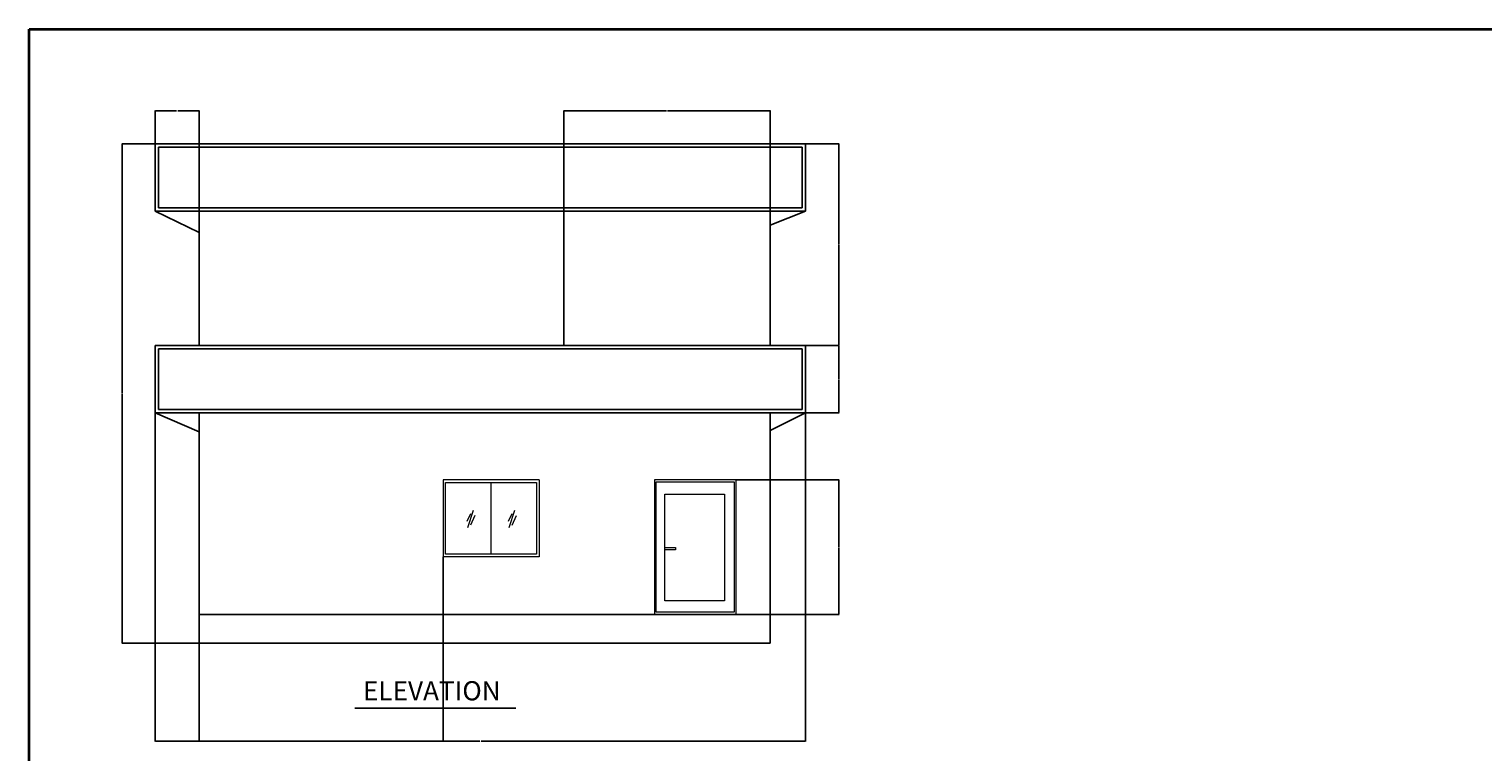
# Model space of a CAD drawing. Units: inches. Extents: x 1912 to 3731, y 1384 to 2459.
# Tile 5 of 8: x 1912 to 2821, y 2007 to 2459. Entities that reach past the tile are written whole.
import ezdxf

# ---------------------------------------------------------------- set-up
doc = ezdxf.new("R2010")
doc.units = ezdxf.units.IN
for name, color, linetype, lineweight in [('A-ANNO-DIMS', 2, 'Continuous', 18), ('A-ANNO-TITL', 7, 'Continuous', 25), ('A-ANNO-TTLB', 7, 'Continuous', 35), ('A-DOOR', 3, 'Continuous', 20), ('A-ELEV', 7, 'Continuous', 25), ('A-GLAZ', 4, 'Continuous', 18)]:
    doc.layers.add(name, color=color, linetype=linetype, lineweight=lineweight)
doc.styles.get("Standard").update_dxf_attribs({"font": 'arial.ttf'})
doc.dimstyles.get("Standard").update_dxf_attribs({"dimtxt": 0.18, "dimasz": 0.18, "dimexe": 0.18, "dimexo": 0.0625, "dimgap": 0.09, "dimtad": 0, "dimtih": 1, "dimtoh": 1, "dimdec": 4, "dimzin": 0, "dimdsep": 46, "dimtxsty": 'Standard', "dimcen": 0.09, "dimadec": 0, "dimazin": 0, "dimtfac": 1, "dimtdec": 4, "dimtofl": 0, "dimtmove": 0, "dimatfit": 3, "dimfxl": 1, "dimtolj": 1, "dimtzin": 0, "dimarcsym": 0})

# ---------------------------------------------------------------- blocks, each defined once
blk = doc.blocks.new('*D115')
at = {"layer": 'A-ANNO-DIMS', "color": 0, "lineweight": -2, "transparency": 16777216}
for p, q in [((1991.12, 2218.67), (1991.12, 2013.22)), ((2397.55, 2218.67), (2397.55, 2013.22)), ((1991.3, 2013.4), (2193.94, 2013.4)), ((2397.37, 2013.4), (2194.73, 2013.4))]:
    blk.add_line(p, q, dxfattribs=at)
at = {"layer": 'A-ANNO-DIMS', "color": 0, "transparency": 16777216}
for points in [[(1991.3, 2013.43), (1991.3, 2013.37), (1991.12, 2013.4)], [(2397.37, 2013.43), (2397.37, 2013.37), (2397.55, 2013.4)]]:
    blk.add_solid(points, dxfattribs=at)
at = {"layer": 'Defpoints', "color": 0, "transparency": 16777216}
for p in [(1991.12, 2218.73), (2397.55, 2218.73), (2397.55, 2013.4)]:
    blk.add_point(p, dxfattribs=at)
at = {"layer": 'A-ANNO-DIMS', "color": 0, "transparency": 16777216, "insert": (2194.33, 2013.4), "char_height": 0.18, "attachment_point": 5}
blk.add_mtext('\\A1;406.4', dxfattribs=at)
blk = doc.blocks.new('*D116')
at = {"layer": 'A-ANNO-DIMS', "color": 0, "lineweight": -2, "transparency": 16777216}
for p, q in [((1991.05, 2386.73), (1970.19, 2386.73)), ((1970.37, 2386.55), (1970.37, 2230.92)), ((1970.37, 2074.91), (1970.37, 2230.55)), ((2018.47, 2074.73), (1970.19, 2074.73))]:
    blk.add_line(p, q, dxfattribs=at)
at = {"layer": 'A-ANNO-DIMS', "color": 0, "transparency": 16777216}
for points in [[(1970.34, 2386.55), (1970.4, 2386.55), (1970.37, 2386.73)], [(1970.34, 2074.91), (1970.4, 2074.91), (1970.37, 2074.73)]]:
    blk.add_solid(points, dxfattribs=at)
at = {"layer": 'Defpoints', "color": 0, "transparency": 16777216}
for p in [(1970.37, 2386.73), (1991.12, 2386.73), (2018.53, 2074.73)]:
    blk.add_point(p, dxfattribs=at)
at = {"layer": 'A-ANNO-DIMS', "color": 0, "transparency": 16777216, "insert": (1970.37, 2230.73), "char_height": 0.18, "attachment_point": 5}
blk.add_mtext('\\A1;312', dxfattribs=at)
blk = doc.blocks.new('*D117')
at = {"layer": 'A-ANNO-DIMS', "color": 0, "lineweight": -2, "transparency": 16777216}
for p, q in [((2171, 2128.67), (2171, 2013.22)), ((2018.53, 2092.67), (2018.53, 2013.22)), ((2018.71, 2013.4), (2094.31, 2013.4)), ((2170.82, 2013.4), (2095.22, 2013.4))]:
    blk.add_line(p, q, dxfattribs=at)
at = {"layer": 'A-ANNO-DIMS', "color": 0, "transparency": 16777216}
for points in [[(2018.71, 2013.43), (2018.71, 2013.37), (2018.53, 2013.4)], [(2170.82, 2013.43), (2170.82, 2013.37), (2171, 2013.4)]]:
    blk.add_solid(points, dxfattribs=at)
at = {"layer": 'Defpoints', "color": 0, "transparency": 16777216}
for p in [(2171, 2128.73), (2018.53, 2092.73), (2171, 2013.4)]:
    blk.add_point(p, dxfattribs=at)
at = {"layer": 'A-ANNO-DIMS', "color": 0, "transparency": 16777216, "insert": (2094.77, 2013.4), "char_height": 0.18, "attachment_point": 5}
blk.add_mtext('\\A1;152.47', dxfattribs=at)
blk = doc.blocks.new('*D118')
at = {"layer": 'A-ANNO-DIMS', "color": 0, "lineweight": -2, "transparency": 16777216}
for p, q in [((2354.01, 2176.73), (2418.48, 2176.73)), ((2418.3, 2176.55), (2418.3, 2134.92)), ((2418.3, 2092.91), (2418.3, 2134.55)), ((2354.01, 2092.73), (2418.48, 2092.73))]:
    blk.add_line(p, q, dxfattribs=at)
at = {"layer": 'A-ANNO-DIMS', "color": 0, "transparency": 16777216}
for points in [[(2418.27, 2176.55), (2418.33, 2176.55), (2418.3, 2176.73)], [(2418.27, 2092.91), (2418.33, 2092.91), (2418.3, 2092.73)]]:
    blk.add_solid(points, dxfattribs=at)
at = {"layer": 'Defpoints', "color": 0, "transparency": 16777216}
for p in [(2353.95, 2176.73), (2418.3, 2176.73), (2353.95, 2092.73)]:
    blk.add_point(p, dxfattribs=at)
at = {"layer": 'A-ANNO-DIMS', "color": 0, "transparency": 16777216, "insert": (2418.3, 2134.73), "char_height": 0.18, "attachment_point": 5}
blk.add_mtext('\\A1;84', dxfattribs=at)
blk = doc.blocks.new('*D119')
at = {"layer": 'A-ANNO-DIMS', "color": 0, "lineweight": -2, "transparency": 16777216}
for p, q in [((2397.61, 2260.73), (2418.48, 2260.73)), ((2418.3, 2260.55), (2418.3, 2239.91)), ((2418.3, 2218.91), (2418.3, 2239.55)), ((2397.61, 2218.73), (2418.48, 2218.73))]:
    blk.add_line(p, q, dxfattribs=at)
at = {"layer": 'A-ANNO-DIMS', "color": 0, "transparency": 16777216}
for points in [[(2418.27, 2260.55), (2418.33, 2260.55), (2418.3, 2260.73)], [(2418.27, 2218.91), (2418.33, 2218.91), (2418.3, 2218.73)]]:
    blk.add_solid(points, dxfattribs=at)
at = {"layer": 'Defpoints', "color": 0, "transparency": 16777216}
for p in [(2397.55, 2260.73), (2418.3, 2260.73), (2397.55, 2218.73)]:
    blk.add_point(p, dxfattribs=at)
at = {"layer": 'A-ANNO-DIMS', "color": 0, "transparency": 16777216, "insert": (2418.3, 2239.73), "char_height": 0.18, "attachment_point": 5}
blk.add_mtext('\\A1;42', dxfattribs=at)
blk = doc.blocks.new('*D120')
at = {"layer": 'A-ANNO-DIMS', "color": 0, "lineweight": -2, "transparency": 16777216}
for p, q in [((2397.61, 2386.73), (2418.48, 2386.73)), ((2418.3, 2386.55), (2418.3, 2323.92)), ((2418.3, 2260.91), (2418.3, 2323.55)), ((2397.61, 2260.73), (2418.48, 2260.73))]:
    blk.add_line(p, q, dxfattribs=at)
at = {"layer": 'A-ANNO-DIMS', "color": 0, "transparency": 16777216}
for points in [[(2418.27, 2386.55), (2418.33, 2386.55), (2418.3, 2386.73)], [(2418.27, 2260.91), (2418.33, 2260.91), (2418.3, 2260.73)]]:
    blk.add_solid(points, dxfattribs=at)
at = {"layer": 'Defpoints', "color": 0, "transparency": 16777216}
for p in [(2397.55, 2386.73), (2418.3, 2386.73), (2397.55, 2260.73)]:
    blk.add_point(p, dxfattribs=at)
at = {"layer": 'A-ANNO-DIMS', "color": 0, "transparency": 16777216, "insert": (2418.3, 2323.73), "char_height": 0.18, "attachment_point": 5}
blk.add_mtext('\\A1;126', dxfattribs=at)
blk = doc.blocks.new('*D121')
at = {"layer": 'A-ANNO-DIMS', "color": 0, "lineweight": -2, "transparency": 16777216}
for p, q in [((2246.53, 2344.8), (2246.53, 2407.66)), ((2246.71, 2407.48), (2310.75, 2407.48)), ((2375.35, 2407.48), (2311.31, 2407.48)), ((2375.53, 2344.8), (2375.53, 2407.66))]:
    blk.add_line(p, q, dxfattribs=at)
at = {"layer": 'A-ANNO-DIMS', "color": 0, "transparency": 16777216}
for points in [[(2246.71, 2407.51), (2246.71, 2407.45), (2246.53, 2407.48)], [(2375.35, 2407.51), (2375.35, 2407.45), (2375.53, 2407.48)]]:
    blk.add_solid(points, dxfattribs=at)
at = {"layer": 'Defpoints', "color": 0, "transparency": 16777216}
for p in [(2375.53, 2407.48), (2246.53, 2344.73), (2375.53, 2344.73)]:
    blk.add_point(p, dxfattribs=at)
at = {"layer": 'A-ANNO-DIMS', "color": 0, "transparency": 16777216, "insert": (2311.03, 2407.48), "char_height": 0.18, "attachment_point": 5}
blk.add_mtext('\\A1;129', dxfattribs=at)
blk = doc.blocks.new('*D122')
at = {"layer": 'A-ANNO-DIMS', "color": 0, "lineweight": -2, "transparency": 16777216}
for p, q in [((1991.12, 2344.8), (1991.12, 2407.66)), ((1991.3, 2407.48), (2004.36, 2407.48)), ((2018.35, 2407.48), (2005.29, 2407.48)), ((2018.53, 2344.8), (2018.53, 2407.66))]:
    blk.add_line(p, q, dxfattribs=at)
at = {"layer": 'A-ANNO-DIMS', "color": 0, "transparency": 16777216}
for points in [[(1991.3, 2407.51), (1991.3, 2407.45), (1991.12, 2407.48)], [(2018.35, 2407.51), (2018.35, 2407.45), (2018.53, 2407.48)]]:
    blk.add_solid(points, dxfattribs=at)
at = {"layer": 'Defpoints', "color": 0, "transparency": 16777216}
for p in [(2018.53, 2407.48), (1991.12, 2344.73), (2018.53, 2344.73)]:
    blk.add_point(p, dxfattribs=at)
at = {"layer": 'A-ANNO-DIMS', "color": 0, "transparency": 16777216, "insert": (2004.82, 2407.48), "char_height": 0.18, "attachment_point": 5}
blk.add_mtext('\\A1;27.414', dxfattribs=at)

msp = doc.modelspace()

# ---------------------------------------------------------------- linework, layer by layer
at = {"layer": 'A-ANNO-TITL'}
msp.add_line((2115.8013, 2034.1548), (2216.5601, 2034.1548), dxfattribs=at)
at = {"layer": 'A-ANNO-TTLB'}
msp.add_lwpolyline([(1912.2029, 2458.5537), (3720.218, 2458.5537), (3720.218, 1383.9599), (1912.2029, 1383.9599)], close=True, dxfattribs=at)
at = {"layer": 'A-DOOR'}
for p, q in [((2303.1185, 2176.7342), (2303.1185, 2092.7342)), ((2353.9519, 2176.7342), (2303.1185, 2176.7342)), ((2353.9519, 2176.7342), (2353.9519, 2092.7342))]:
    msp.add_line(p, q, dxfattribs=at)
for points in [[(2304.1765, 2175.5605), (2352.8636, 2175.5605), (2352.8636, 2094.1028), (2304.1765, 2094.1028)], [(2309.576, 2167.7922), (2346.9489, 2167.7922), (2346.9489, 2101.1483), (2309.576, 2101.1483)], [(2309.576, 2134.4702), (2316.312, 2134.4702), (2316.312, 2133.1152), (2309.576, 2133.1152)]]:
    msp.add_lwpolyline(points, close=True, dxfattribs=at)
at = {"layer": 'A-ELEV'}
for p, q in [((2397.5474, 2386.7342), (1991.1167, 2386.7342)), ((1991.1167, 2344.7342), (1991.1167, 2386.7342)), ((1991.1167, 2386.7342), (1991.1167, 2384.7342)), ((1993.1167, 2384.7342), (2395.5474, 2384.7342)), ((1993.1167, 2346.7342), (1993.1167, 2384.7342)), ((2395.5474, 2384.7342), (2395.5474, 2346.7342)), ((2397.5474, 2344.7342), (2397.5474, 2386.7342)), ((2397.5474, 2344.7342), (1991.1167, 2344.7342)), ((1991.1167, 2344.7342), (2018.5308, 2331.3913)), ((2395.5474, 2346.7342), (1993.1167, 2346.7342)), ((2018.5308, 2344.7342), (2018.5308, 2260.7342)), ((2246.5308, 2344.7342), (2246.5308, 2260.7342)), ((2375.5308, 2344.7342), (2375.5308, 2260.7342)), ((2397.5474, 2344.7342), (2375.5308, 2336.0444)), ((2018.5308, 2331.3913), (2018.5308, 2331.3913)), ((2397.5474, 2260.7342), (1991.1167, 2260.7342)), ((1991.1167, 2218.7342), (1991.1167, 2260.7342)), ((2395.5474, 2258.7342), (1993.1167, 2258.7342)), ((1993.1167, 2258.7342), (1993.1167, 2220.7342)), ((2395.5474, 2220.7342), (2395.5474, 2258.7342)), ((2397.5474, 2218.7342), (2397.5474, 2260.7342)), ((2397.5474, 2260.7342), (2397.5474, 2258.7342)), ((2397.5474, 2218.7342), (1991.1167, 2218.7342)), ((1991.1167, 2218.7342), (2018.5308, 2206.7463)), ((1993.1167, 2220.7342), (2395.5474, 2220.7342)), ((2018.5308, 2218.7342), (2018.5308, 2074.7342)), ((2018.5308, 2218.7342), (2018.5308, 2200.7342)), ((2375.5308, 2218.7342), (2375.5308, 2074.7342)), ((2375.5308, 2218.7342), (2375.5308, 2200.7342)), ((2397.5474, 2218.7342), (2375.5308, 2207.6524)), ((2375.5308, 2092.7342), (2018.5308, 2092.7342)), ((2375.5308, 2074.7342), (2018.5308, 2074.7342))]:
    msp.add_line(p, q, dxfattribs=at)
at = {"layer": 'A-GLAZ'}
for p, q in [((2171.0029, 2176.7342), (2171.0029, 2128.7342)), ((2231.0029, 2176.7342), (2171.0029, 2176.7342)), ((2200.9445, 2175.1331), (2200.9445, 2130.3412)), ((2231.0029, 2176.7342), (2231.0029, 2128.7342)), ((2188.046, 2155.5362), (2185.8984, 2150.816)), ((2189.7101, 2157.6336), (2186.1807, 2146.8965)), ((2190.7745, 2154.4632), (2188.1801, 2148.4442)), ((2213.8955, 2155.4564), (2211.7479, 2150.7362)), ((2215.5596, 2157.5538), (2212.0302, 2146.8166)), ((2216.624, 2154.3834), (2214.0296, 2148.3643)), ((2231.0029, 2128.7342), (2171.0029, 2128.7342))]:
    msp.add_line(p, q, dxfattribs=at)
msp.add_lwpolyline([(2172.5227, 2175.1331), (2229.3663, 2175.1331), (2229.3663, 2130.3412), (2172.5227, 2130.3412)], close=True, dxfattribs=at)

# ---------------------------------------------------------------- texts
at = {"layer": 'A-ANNO-TITL', "insert": (2120.8784, 2050.965), "char_height": 12, "attachment_point": 1}
msp.add_mtext_dynamic_manual_height_columns('ELEVATION', width=351.7799, gutter_width=12.5, heights=[0], dxfattribs=at)

# ---------------------------------------------------------------- dimensions: what is measured, and where the dimension line sits
at = {"layer": 'A-ANNO-DIMS'}
for base, p1, p2, override, picture, middle in [((2018.5308, 2407.4842), (1991.1167, 2344.7342), (2018.5308, 2344.7342), {"dimdec": 3, "dimlfac": 1, "dimrnd": 0, "dimzin": 0, "dimdsep": 46, "dimlunit": 2}, '*D122', (2004.8237, 2407.4842)), ((2375.5308, 2407.4842), (2246.5308, 2344.7342), (2375.5308, 2344.7342), {"dimdec": 0, "dimlfac": 1, "dimrnd": 0, "dimzin": 0, "dimdsep": 46, "dimlunit": 2}, '*D121', (2311.0308, 2407.4842)), ((2397.5474, 2013.4048), (1991.1167, 2218.7342), (2397.5474, 2218.7342), {"dimdec": 1, "dimlfac": 1, "dimrnd": 0, "dimzin": 0, "dimdsep": 46, "dimlunit": 2}, '*D115', (2194.332, 2013.4048)), ((2171.0029, 2013.4048), (2018.5308, 2092.7342), (2171.0029, 2128.7342), {"dimdec": 2, "dimlfac": 1, "dimrnd": 0, "dimzin": 0, "dimdsep": 46, "dimlunit": 2}, '*D117', (2094.7668, 2013.4048))]:
    dim = msp.add_linear_dim(base=base, p1=p1, p2=p2, dimstyle='Standard', override=override, dxfattribs=at)
    dim.commit()
    dim.dimension.update_dxf_attribs({"geometry": picture, "text_midpoint": middle})
for base, p1, p2, picture, middle in [((1970.3667, 2386.7342), (2018.5308, 2074.7342), (1991.1167, 2386.7342), '*D116', (1970.3667, 2230.7342)), ((2418.2974, 2386.7342), (2397.5474, 2260.7342), (2397.5474, 2386.7342), '*D120', (2418.2974, 2323.7342)), ((2418.2974, 2260.7342), (2397.5474, 2218.7342), (2397.5474, 2260.7342), '*D119', (2418.2974, 2239.7342)), ((2418.2974, 2176.7342), (2353.9519, 2092.7342), (2353.9519, 2176.7342), '*D118', (2418.2974, 2134.7342))]:
    dim = msp.add_linear_dim(base=base, p1=p1, p2=p2, angle=90, dimstyle='Standard', override={"dimdec": 0, "dimlfac": 1, "dimrnd": 0, "dimzin": 0, "dimdsep": 46, "dimlunit": 2}, dxfattribs=at)
    dim.commit()
    dim.dimension.update_dxf_attribs({"geometry": picture, "text_midpoint": middle})

doc.saveas('drawing.dxf')
